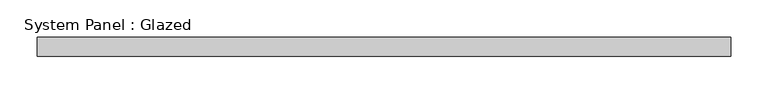
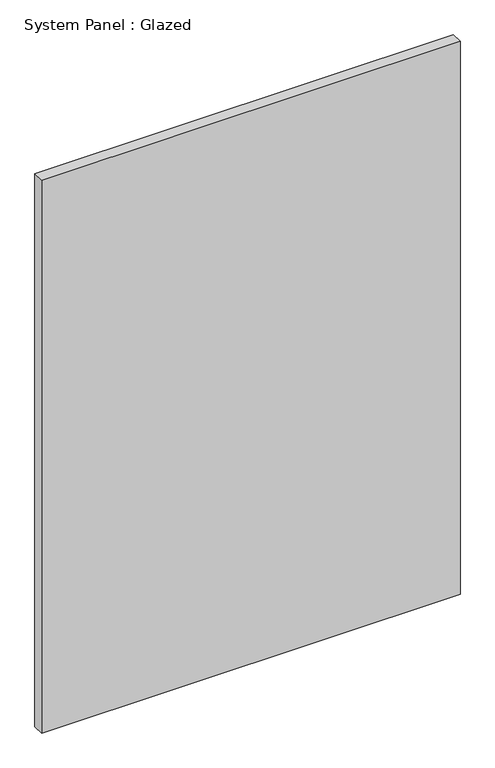
"""IFC4 building model written with IfcOpenShell, lengths in millimetres: plate geometry, System Panel : Glazed."""

from ifc_helpers import new_model, si_unit, origin, origin_with_axes, place, context, project, spatial, polyline, outline, extrude, source, transform, mapped, element, save


def system_panel_glazed_5df0e43d(model_context):
    return source(origin(), model_context, "Body", "SweptSolid", [
        extrude(outline(polyline([(463.55, 19.05), (-463.55, 19.05), (-463.55, 44.45), (463.55, 44.45), (463.55, 19.05)])), origin_with_axes(), (0.0, 0.0, 1.0), 1295.1292854),
    ])


if __name__ == "__main__":
    model = new_model("IFC4")
    model_context = context("Model", 3, world=origin())
    ifc_project = project(units=[si_unit("LENGTHUNIT", "METRE", prefix="MILLI")], contexts=[model_context])
    site = spatial("IfcSite", under=ifc_project)
    building = spatial("IfcBuilding", under=site)
    placement = place(None, origin())
    system_panel_glazed_shape = system_panel_glazed_5df0e43d(model_context)
    element("IfcPlate", 1, ObjectType="System Panel : Glazed", at=placement, inside=building, context=model_context, shape_type="MappedRepresentation", body=[
        mapped(system_panel_glazed_shape, transform((0.0, 0.0, 0.0), x_axis=(1.0, 0.0, 0.0), y_axis=(0.0, 1.0, 0.0), z_axis=(0.0, 0.0, 1.0))),
    ])
    save(model, "model.ifc")

# Revit data of these elements
# Type "System Panel : Glazed"
#   Construction Type Id = "GSP4R"
#   Analytic Construction = "1/8 in Pilkington single glazing"
#   Visual Light Transmittance = 0.9
#   Solar Heat Gain Coefficient = 0.86
#   Heat Transfer Coefficient (U) = 1.18115 BTU/(h·ft²·°F)
#   Define Thermal Properties by = 1
# Element 1 (IfcPlate, "System Panel : Glazed")
#   Materials on its faces: "Glass"
# Materials
#   "Glass": class "Glass", colour RGB 0 128 192, transparency 0.75, Description = "Soda Lime Glass", Cost = 0
